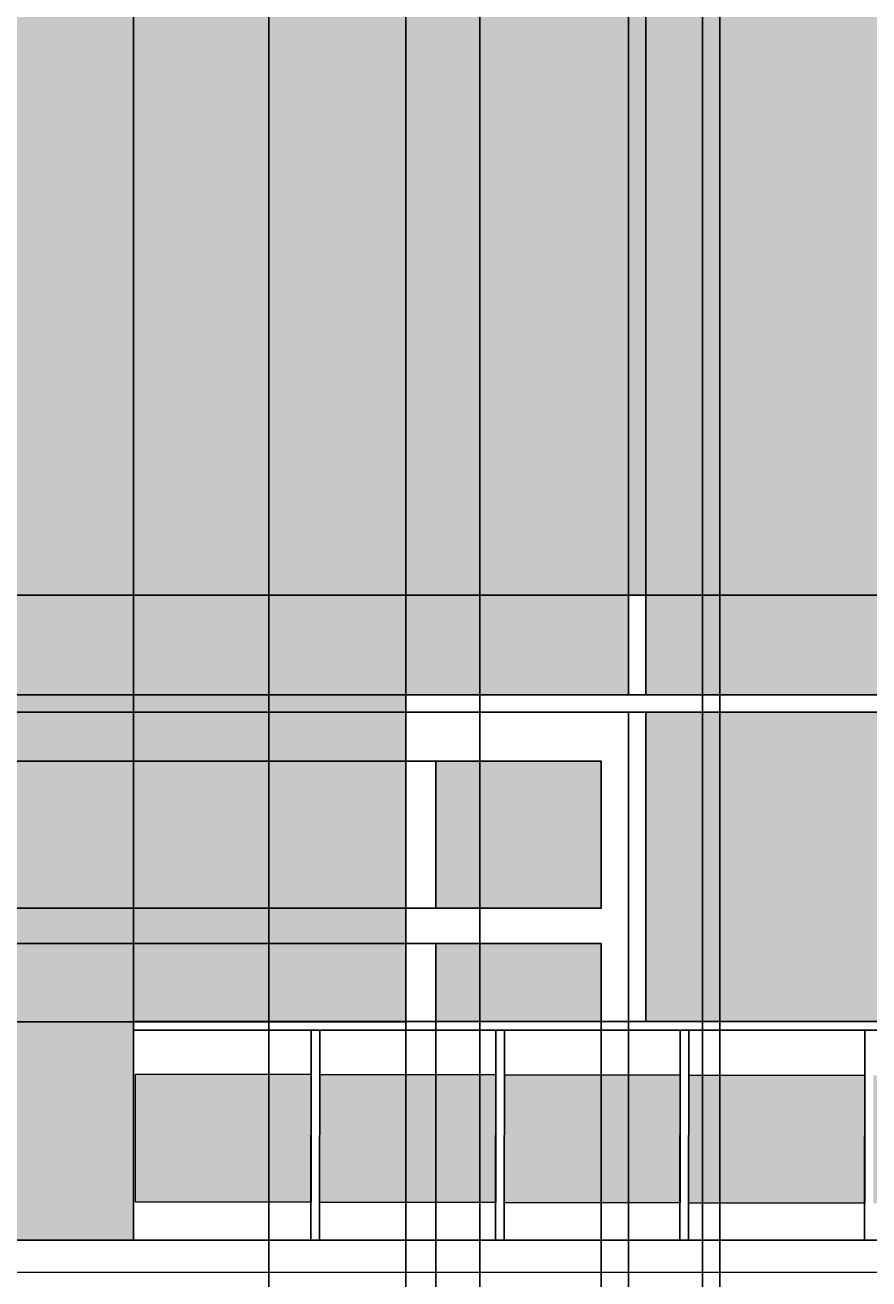
# Model space of a CAD drawing. Units: inches. Extents: x 36 to 594, y 79 to 831.
# Tile 18 of 30: x 189 to 286, y 446 to 590. Entities that reach past the tile are written whole.
import ezdxf

# ---------------------------------------------------------------- set-up
doc = ezdxf.new("R2010")
doc.units = ezdxf.units.IN
doc.header["$MEASUREMENT"] = 0
for name, color, linetype, lineweight in [('A-ANNO-DIMS', 2, 'Continuous', 18), ('A-ELEV', 7, 'Continuous', 25), ('A-ELEV-PATT', 8, 'Continuous', 13), ('A-GLAZ', 4, 'Continuous', 18)]:
    doc.layers.add(name, color=color, linetype=linetype, lineweight=lineweight)
doc.styles.get("Standard").update_dxf_attribs({"font": 'arial.ttf'})
doc.dimstyles.get("Standard").update_dxf_attribs({"dimtxt": 0.8125, "dimasz": 0.18, "dimexe": 0.18, "dimexo": 0.0625, "dimgap": 0.09, "dimtad": 0, "dimtih": 1, "dimtoh": 1, "dimdec": 4, "dimzin": 0, "dimdsep": 46, "dimlunit": 4, "dimtxsty": 'Standard', "dimcen": 0.09, "dimadec": 0, "dimazin": 0, "dimtfac": 1, "dimtdec": 4, "dimtofl": 0, "dimtmove": 0, "dimatfit": 3, "dimfxl": 1, "dimtolj": 1, "dimtzin": 0, "dimarcsym": 0})

# ---------------------------------------------------------------- blocks, each defined once
blk = doc.blocks.new('GLAZ-PANEL')
blk.add_lwpolyline([(0, 14.77), (20.28, 14.77), (20.28, 0), (0, 0)], close=True)
blk = doc.blocks.new('*D28')
at = {"layer": 'A-ANNO-DIMS', "color": 0, "lineweight": -2, "transparency": 16777216}
for p, q in [((269.3, 796.05), (37.49, 796.05)), ((37.67, 795.87), (37.67, 455.63)), ((37.67, 114.39), (37.67, 454.62)), ((94.8, 114.21), (37.49, 114.21))]:
    blk.add_line(p, q, dxfattribs=at)
at = {"layer": 'A-ANNO-DIMS', "color": 0, "transparency": 16777216}
for points in [[(37.64, 795.87), (37.7, 795.87), (37.67, 796.05)], [(37.64, 114.39), (37.7, 114.39), (37.67, 114.21)]]:
    blk.add_solid(points, dxfattribs=at)
at = {"layer": 'Defpoints', "color": 0, "transparency": 16777216}
for p in [(37.67, 796.05), (269.36, 796.05), (94.87, 114.21)]:
    blk.add_point(p, dxfattribs=at)
at = {"layer": 'A-ANNO-DIMS', "color": 0, "transparency": 16777216, "insert": (37.67, 455.13), "char_height": 0.812, "attachment_point": 5}
blk.add_mtext('\\A1;681.8', dxfattribs=at)
blk = doc.blocks.new('*D61')
at = {"layer": 'A-ANNO-DIMS', "color": 0, "lineweight": -2, "transparency": 16777216}
for p, q in [((156.41, 264.68), (156.41, 830.73)), ((156.59, 830.55), (185.26, 830.55)), ((216.85, 830.55), (188.18, 830.55)), ((217.03, 286.24), (217.03, 830.73))]:
    blk.add_line(p, q, dxfattribs=at)
at = {"layer": 'A-ANNO-DIMS', "color": 0, "transparency": 16777216}
for points in [[(156.59, 830.58), (156.59, 830.52), (156.41, 830.55)], [(216.85, 830.58), (216.85, 830.52), (217.03, 830.55)]]:
    blk.add_solid(points, dxfattribs=at)
at = {"layer": 'Defpoints', "color": 0, "transparency": 16777216}
for p in [(217.03, 830.55), (217.03, 286.18), (156.41, 264.62)]:
    blk.add_point(p, dxfattribs=at)
at = {"layer": 'A-ANNO-DIMS', "color": 0, "transparency": 16777216, "insert": (186.72, 830.55), "char_height": 0.812, "attachment_point": 5}
blk.add_mtext('\\A1;60.62', dxfattribs=at)
blk = doc.blocks.new('*D92')
at = {"layer": 'A-ANNO-DIMS', "color": 0, "lineweight": -2, "transparency": 16777216}
for p, q in [((201.42, 475.48), (201.42, 830.73)), ((201.6, 830.55), (215.98, 830.55)), ((232.64, 830.55), (218.26, 830.55)), ((232.82, 524.67), (232.82, 830.73))]:
    blk.add_line(p, q, dxfattribs=at)
at = {"layer": 'A-ANNO-DIMS', "color": 0, "transparency": 16777216}
for points in [[(201.6, 830.58), (201.6, 830.52), (201.42, 830.55)], [(232.64, 830.58), (232.64, 830.52), (232.82, 830.55)]]:
    blk.add_solid(points, dxfattribs=at)
at = {"layer": 'Defpoints', "color": 0, "transparency": 16777216}
for p in [(232.82, 830.55), (232.82, 524.6), (201.42, 475.41)]:
    blk.add_point(p, dxfattribs=at)
at = {"layer": 'A-ANNO-DIMS', "color": 0, "transparency": 16777216, "insert": (217.12, 830.55), "char_height": 0.812, "attachment_point": 5}
blk.add_mtext('\\A1;31.4', dxfattribs=at)
blk = doc.blocks.new('*D93')
at = {"layer": 'A-ANNO-DIMS', "color": 0, "lineweight": -2, "transparency": 16777216}
for p, q in [((232.82, 524.67), (232.82, 830.73)), ((233, 830.55), (243.88, 830.55)), ((258.33, 830.55), (247.45, 830.55)), ((258.51, 524.67), (258.51, 830.73))]:
    blk.add_line(p, q, dxfattribs=at)
at = {"layer": 'A-ANNO-DIMS', "color": 0, "transparency": 16777216}
for points in [[(233, 830.58), (233, 830.52), (232.82, 830.55)], [(258.33, 830.58), (258.33, 830.52), (258.51, 830.55)]]:
    blk.add_solid(points, dxfattribs=at)
at = {"layer": 'Defpoints', "color": 0, "transparency": 16777216}
for p in [(258.51, 830.55), (232.82, 524.6), (258.51, 524.6)]:
    blk.add_point(p, dxfattribs=at)
at = {"layer": 'A-ANNO-DIMS', "color": 0, "transparency": 16777216, "insert": (245.66, 830.55), "char_height": 0.812, "attachment_point": 5}
blk.add_mtext('\\A1;25.684', dxfattribs=at)
blk = doc.blocks.new('*D94')
at = {"layer": 'A-ANNO-DIMS', "color": 0, "lineweight": -2, "transparency": 16777216}
for p, q in [((258.51, 524.67), (258.51, 830.73)), ((258.69, 830.55), (259.15, 830.55)), ((260.33, 830.55), (259.86, 830.55)), ((260.51, 524.67), (260.51, 830.73))]:
    blk.add_line(p, q, dxfattribs=at)
at = {"layer": 'A-ANNO-DIMS', "color": 0, "transparency": 16777216}
for points in [[(258.69, 830.58), (258.69, 830.52), (258.51, 830.55)], [(260.33, 830.58), (260.33, 830.52), (260.51, 830.55)]]:
    blk.add_solid(points, dxfattribs=at)
at = {"layer": 'Defpoints', "color": 0, "transparency": 16777216}
for p in [(260.51, 830.55), (258.51, 524.6), (260.51, 524.6)]:
    blk.add_point(p, dxfattribs=at)
at = {"layer": 'A-ANNO-DIMS', "color": 0, "transparency": 16777216, "insert": (259.51, 830.55), "char_height": 0.812, "attachment_point": 5}
blk.add_mtext('\\A1;2', dxfattribs=at)
blk = doc.blocks.new('*D95')
at = {"layer": 'A-ANNO-DIMS', "color": 0, "lineweight": -2, "transparency": 16777216}
for p, q in [((260.51, 524.67), (260.51, 830.73)), ((260.69, 830.55), (299.71, 830.55)), ((341.66, 830.55), (302.63, 830.55)), ((341.84, 524.67), (341.84, 830.73))]:
    blk.add_line(p, q, dxfattribs=at)
at = {"layer": 'A-ANNO-DIMS', "color": 0, "transparency": 16777216}
for points in [[(260.69, 830.58), (260.69, 830.52), (260.51, 830.55)], [(341.66, 830.58), (341.66, 830.52), (341.84, 830.55)]]:
    blk.add_solid(points, dxfattribs=at)
at = {"layer": 'Defpoints', "color": 0, "transparency": 16777216}
for p in [(341.84, 830.55), (260.51, 524.6), (341.84, 524.6)]:
    blk.add_point(p, dxfattribs=at)
at = {"layer": 'A-ANNO-DIMS', "color": 0, "transparency": 16777216, "insert": (301.17, 830.55), "char_height": 0.812, "attachment_point": 5}
blk.add_mtext('\\A1;81.33', dxfattribs=at)
blk = doc.blocks.new('*D96')
at = {"layer": 'A-ANNO-DIMS', "color": 0, "lineweight": -2, "transparency": 16777216}
for p, q in [((236.29, 484.36), (236.29, 79.53)), ((232.82, 475.35), (232.82, 79.53)), ((233, 79.71), (233.41, 79.71)), ((236.11, 79.71), (235.7, 79.71))]:
    blk.add_line(p, q, dxfattribs=at)
at = {"layer": 'A-ANNO-DIMS', "color": 0, "transparency": 16777216}
for points in [[(233, 79.74), (233, 79.68), (232.82, 79.71)], [(236.11, 79.74), (236.11, 79.68), (236.29, 79.71)]]:
    blk.add_solid(points, dxfattribs=at)
at = {"layer": 'Defpoints', "color": 0, "transparency": 16777216}
for p in [(236.29, 484.42), (232.82, 475.41), (236.29, 79.71)]:
    blk.add_point(p, dxfattribs=at)
at = {"layer": 'A-ANNO-DIMS', "color": 0, "transparency": 16777216, "insert": (234.56, 79.71), "char_height": 0.812, "attachment_point": 5}
blk.add_mtext('\\A1;3.47', dxfattribs=at)
blk = doc.blocks.new('*D97')
at = {"layer": 'A-ANNO-DIMS', "color": 0, "lineweight": -2, "transparency": 16777216}
for p, q in [((236.29, 484.36), (236.29, 79.53)), ((255.36, 484.36), (255.36, 79.53)), ((236.47, 79.71), (244.09, 79.71)), ((255.18, 79.71), (247.56, 79.71))]:
    blk.add_line(p, q, dxfattribs=at)
at = {"layer": 'A-ANNO-DIMS', "color": 0, "transparency": 16777216}
for points in [[(236.47, 79.74), (236.47, 79.68), (236.29, 79.71)], [(255.18, 79.74), (255.18, 79.68), (255.36, 79.71)]]:
    blk.add_solid(points, dxfattribs=at)
at = {"layer": 'Defpoints', "color": 0, "transparency": 16777216}
for p in [(236.29, 484.42), (255.36, 484.42), (255.36, 79.71)]:
    blk.add_point(p, dxfattribs=at)
at = {"layer": 'A-ANNO-DIMS', "color": 0, "transparency": 16777216, "insert": (245.82, 79.71), "char_height": 0.812, "attachment_point": 5}
blk.add_mtext('\\A1;19.064', dxfattribs=at)
blk = doc.blocks.new('*D98')
at = {"layer": 'A-ANNO-DIMS', "color": 0, "lineweight": -2, "transparency": 16777216}
for p, q in [((255.36, 484.36), (255.36, 79.53)), ((258.51, 475.35), (258.51, 79.53)), ((255.54, 79.71), (255.78, 79.71)), ((258.33, 79.71), (258.08, 79.71))]:
    blk.add_line(p, q, dxfattribs=at)
at = {"layer": 'A-ANNO-DIMS', "color": 0, "transparency": 16777216}
for points in [[(255.54, 79.74), (255.54, 79.68), (255.36, 79.71)], [(258.33, 79.74), (258.33, 79.68), (258.51, 79.71)]]:
    blk.add_solid(points, dxfattribs=at)
at = {"layer": 'Defpoints', "color": 0, "transparency": 16777216}
for p in [(255.36, 484.42), (258.51, 475.41), (258.51, 79.71)]:
    blk.add_point(p, dxfattribs=at)
at = {"layer": 'A-ANNO-DIMS', "color": 0, "transparency": 16777216, "insert": (256.93, 79.71), "char_height": 0.812, "attachment_point": 5}
blk.add_mtext('\\A1;3.15', dxfattribs=at)
blk = doc.blocks.new('*D99')
at = {"layer": 'A-ANNO-DIMS', "color": 0, "lineweight": -2, "transparency": 16777216}
for p, q in [((236.23, 484.42), (37.49, 484.42)), ((37.67, 484.24), (37.67, 480.42)), ((37.67, 475.59), (37.67, 479.41)), ((232.76, 475.41), (37.49, 475.41))]:
    blk.add_line(p, q, dxfattribs=at)
at = {"layer": 'A-ANNO-DIMS', "color": 0, "transparency": 16777216}
for points in [[(37.64, 484.24), (37.7, 484.24), (37.67, 484.42)], [(37.64, 475.59), (37.7, 475.59), (37.67, 475.41)]]:
    blk.add_solid(points, dxfattribs=at)
at = {"layer": 'Defpoints', "color": 0, "transparency": 16777216}
for p in [(37.67, 484.42), (236.29, 484.42), (232.82, 475.41)]:
    blk.add_point(p, dxfattribs=at)
at = {"layer": 'A-ANNO-DIMS', "color": 0, "transparency": 16777216, "insert": (37.67, 479.92), "char_height": 0.812, "attachment_point": 5}
blk.add_mtext('\\A1;9.005', dxfattribs=at)
blk = doc.blocks.new('*D100')
at = {"layer": 'A-ANNO-DIMS', "color": 0, "lineweight": -2, "transparency": 16777216}
for p, q in [((236.23, 488.49), (37.49, 488.49)), ((37.67, 488.31), (37.67, 486.96)), ((37.67, 484.6), (37.67, 485.95)), ((236.23, 484.42), (37.49, 484.42))]:
    blk.add_line(p, q, dxfattribs=at)
at = {"layer": 'A-ANNO-DIMS', "color": 0, "transparency": 16777216}
for points in [[(37.64, 488.31), (37.7, 488.31), (37.67, 488.49)], [(37.64, 484.6), (37.7, 484.6), (37.67, 484.42)]]:
    blk.add_solid(points, dxfattribs=at)
at = {"layer": 'Defpoints', "color": 0, "transparency": 16777216}
for p in [(37.67, 488.49), (236.29, 488.49), (236.29, 484.42)]:
    blk.add_point(p, dxfattribs=at)
at = {"layer": 'A-ANNO-DIMS', "color": 0, "transparency": 16777216, "insert": (37.67, 486.46), "char_height": 0.812, "attachment_point": 5}
blk.add_mtext('\\A1;4.074', dxfattribs=at)
blk = doc.blocks.new('*D101')
at = {"layer": 'A-ANNO-DIMS', "color": 0, "lineweight": -2, "transparency": 16777216}
for p, q in [((236.23, 505.45), (37.49, 505.45)), ((37.67, 505.27), (37.67, 497.48)), ((37.67, 488.67), (37.67, 496.47)), ((236.23, 488.49), (37.49, 488.49))]:
    blk.add_line(p, q, dxfattribs=at)
at = {"layer": 'A-ANNO-DIMS', "color": 0, "transparency": 16777216}
for points in [[(37.64, 505.27), (37.7, 505.27), (37.67, 505.45)], [(37.64, 488.67), (37.7, 488.67), (37.67, 488.49)]]:
    blk.add_solid(points, dxfattribs=at)
at = {"layer": 'Defpoints', "color": 0, "transparency": 16777216}
for p in [(37.67, 505.45), (236.29, 505.45), (236.29, 488.49)]:
    blk.add_point(p, dxfattribs=at)
at = {"layer": 'A-ANNO-DIMS', "color": 0, "transparency": 16777216, "insert": (37.67, 496.97), "char_height": 0.812, "attachment_point": 5}
blk.add_mtext('\\A1;16.957', dxfattribs=at)
blk = doc.blocks.new('*D102')
at = {"layer": 'A-ANNO-DIMS', "color": 0, "lineweight": -2, "transparency": 16777216}
for p, q in [((232.76, 511.12), (37.49, 511.12)), ((37.67, 510.94), (37.67, 508.79)), ((37.67, 505.63), (37.67, 507.78)), ((236.23, 505.45), (37.49, 505.45))]:
    blk.add_line(p, q, dxfattribs=at)
at = {"layer": 'A-ANNO-DIMS', "color": 0, "transparency": 16777216}
for points in [[(37.64, 510.94), (37.7, 510.94), (37.67, 511.12)], [(37.64, 505.63), (37.7, 505.63), (37.67, 505.45)]]:
    blk.add_solid(points, dxfattribs=at)
at = {"layer": 'Defpoints', "color": 0, "transparency": 16777216}
for p in [(37.67, 511.12), (232.82, 511.12), (236.29, 505.45)]:
    blk.add_point(p, dxfattribs=at)
at = {"layer": 'A-ANNO-DIMS', "color": 0, "transparency": 16777216, "insert": (37.67, 508.29), "char_height": 0.812, "attachment_point": 5}
blk.add_mtext('\\A1;5.672', dxfattribs=at)
blk = doc.blocks.new('*D103')
at = {"layer": 'A-ANNO-DIMS', "color": 0, "lineweight": -2, "transparency": 16777216}
for p, q in [((232.76, 513.12), (37.49, 513.12)), ((37.67, 512.94), (37.67, 512.62)), ((232.76, 511.12), (37.49, 511.12)), ((37.67, 511.3), (37.67, 511.62))]:
    blk.add_line(p, q, dxfattribs=at)
at = {"layer": 'A-ANNO-DIMS', "color": 0, "transparency": 16777216}
for points in [[(37.64, 512.94), (37.7, 512.94), (37.67, 513.12)], [(37.64, 511.3), (37.7, 511.3), (37.67, 511.12)]]:
    blk.add_solid(points, dxfattribs=at)
at = {"layer": 'Defpoints', "color": 0, "transparency": 16777216}
for p in [(37.67, 513.12), (232.82, 513.12), (232.82, 511.12)]:
    blk.add_point(p, dxfattribs=at)
at = {"layer": 'A-ANNO-DIMS', "color": 0, "transparency": 16777216, "insert": (37.67, 512.12), "char_height": 0.812, "attachment_point": 5}
blk.add_mtext('\\A1;2', dxfattribs=at)
blk = doc.blocks.new('*D104')
at = {"layer": 'A-ANNO-DIMS', "color": 0, "lineweight": -2, "transparency": 16777216}
for p, q in [((232.76, 524.6), (37.49, 524.6)), ((37.67, 524.42), (37.67, 519.37)), ((37.67, 513.3), (37.67, 518.36)), ((232.76, 513.12), (37.49, 513.12))]:
    blk.add_line(p, q, dxfattribs=at)
at = {"layer": 'A-ANNO-DIMS', "color": 0, "transparency": 16777216}
for points in [[(37.64, 524.42), (37.7, 524.42), (37.67, 524.6)], [(37.64, 513.3), (37.7, 513.3), (37.67, 513.12)]]:
    blk.add_solid(points, dxfattribs=at)
at = {"layer": 'Defpoints', "color": 0, "transparency": 16777216}
for p in [(37.67, 524.6), (232.82, 524.6), (232.82, 513.12)]:
    blk.add_point(p, dxfattribs=at)
at = {"layer": 'A-ANNO-DIMS', "color": 0, "transparency": 16777216, "insert": (37.67, 518.86), "char_height": 0.812, "attachment_point": 5}
blk.add_mtext('\\A1;11.481', dxfattribs=at)
blk = doc.blocks.new('*D105')
at = {"layer": 'A-ANNO-DIMS', "color": 0, "lineweight": -2, "transparency": 16777216}
for p, q in [((241.36, 404.34), (241.36, 830.73)), ((241.54, 830.55), (252.42, 830.55)), ((266.86, 830.55), (255.98, 830.55)), ((267.04, 404.34), (267.04, 830.73))]:
    blk.add_line(p, q, dxfattribs=at)
at = {"layer": 'A-ANNO-DIMS', "color": 0, "transparency": 16777216}
for points in [[(241.54, 830.58), (241.54, 830.52), (241.36, 830.55)], [(266.86, 830.58), (266.86, 830.52), (267.04, 830.55)]]:
    blk.add_solid(points, dxfattribs=at)
at = {"layer": 'Defpoints', "color": 0, "transparency": 16777216}
for p in [(267.04, 830.55), (241.36, 404.27), (267.04, 404.27)]:
    blk.add_point(p, dxfattribs=at)
at = {"layer": 'A-ANNO-DIMS', "color": 0, "transparency": 16777216, "insert": (254.2, 830.55), "char_height": 0.812, "attachment_point": 5}
blk.add_mtext('\\A1;25.684', dxfattribs=at)
blk = doc.blocks.new('*D106')
at = {"layer": 'A-ANNO-DIMS', "color": 0, "lineweight": -2, "transparency": 16777216}
for p, q in [((267.04, 404.34), (267.04, 830.73)), ((267.22, 830.55), (267.68, 830.55)), ((268.86, 830.55), (268.4, 830.55)), ((269.04, 404.34), (269.04, 830.73))]:
    blk.add_line(p, q, dxfattribs=at)
at = {"layer": 'A-ANNO-DIMS', "color": 0, "transparency": 16777216}
for points in [[(267.22, 830.58), (267.22, 830.52), (267.04, 830.55)], [(268.86, 830.58), (268.86, 830.52), (269.04, 830.55)]]:
    blk.add_solid(points, dxfattribs=at)
at = {"layer": 'Defpoints', "color": 0, "transparency": 16777216}
for p in [(269.04, 830.55), (267.04, 404.27), (269.04, 404.27)]:
    blk.add_point(p, dxfattribs=at)
at = {"layer": 'A-ANNO-DIMS', "color": 0, "transparency": 16777216, "insert": (268.04, 830.55), "char_height": 0.812, "attachment_point": 5}
blk.add_mtext('\\A1;2', dxfattribs=at)
blk = doc.blocks.new('*D107')
at = {"layer": 'A-ANNO-DIMS', "color": 0, "lineweight": -2, "transparency": 16777216}
for p, q in [((269.04, 404.34), (269.04, 830.73)), ((269.22, 830.55), (310.99, 830.55)), ((355.68, 830.55), (313.91, 830.55)), ((355.86, 404.34), (355.86, 830.73))]:
    blk.add_line(p, q, dxfattribs=at)
at = {"layer": 'A-ANNO-DIMS', "color": 0, "transparency": 16777216}
for points in [[(269.22, 830.58), (269.22, 830.52), (269.04, 830.55)], [(355.68, 830.58), (355.68, 830.52), (355.86, 830.55)]]:
    blk.add_solid(points, dxfattribs=at)
at = {"layer": 'Defpoints', "color": 0, "transparency": 16777216}
for p in [(355.86, 830.55), (269.04, 404.27), (355.86, 404.27)]:
    blk.add_point(p, dxfattribs=at)
at = {"layer": 'A-ANNO-DIMS', "color": 0, "transparency": 16777216, "insert": (312.45, 830.55), "char_height": 0.812, "attachment_point": 5}
blk.add_mtext('\\A1;86.82', dxfattribs=at)

msp = doc.modelspace()

# ---------------------------------------------------------------- hatches: boundary and pattern name
at = {"layer": 'A-ELEV-PATT'}
h = msp.add_hatch(color=256, dxfattribs=at)
h.dxf.hatch_style = 1
h.paths.add_polyline_path([(398.0873, 796.0465), (269.3592, 796.0465), (269.3592, 770.1455), (397.8159, 770.1455)])
h.paths.add_polyline_path([(397.7518, 764.0341), (269.3592, 764.0341), (269.3592, 630.0394), (341.8367, 630.0394), (341.8367, 720.595), (335.0881, 728.3699), (329.982, 735.3373), (345.3661, 727.7743), (397.1052, 702.3389)])
h.paths.add_polyline_path([(341.8367, 594.2124), (201.4189, 594.2124), (201.4189, 475.4136), (232.8216, 475.4136), (232.8216, 524.6037), (341.8367, 524.6037)])
h.paths.add_polyline_path([(177.525, 594.2124), (118.7598, 594.2124), (118.7598, 450.2124), (177.525, 450.2124)])
h.paths.add_polyline_path([(424.4958, 594.2124), (365.7306, 594.2124), (365.7306, 450.2124), (424.4958, 450.2124)])
h.paths.add_polyline_path([(241.3553, 404.2737), (355.8569, 404.2737), (355.8569, 355.0836), (424.5492, 355.0836), (424.5492, 425.7333), (118.7598, 426.2844), (118.7598, 355.0836), (241.3553, 355.0836)])
h.paths.add_polyline_path([(448.3898, 306.2124), (217.0273, 306.2124), (217.0273, 142.2124), (254.0293, 142.2124), (254.0293, 150.9347), (254.0293, 286.1802), (401.5491, 286.1802), (401.5491, 150.9347), (401.5491, 142.2124), (448.3898, 142.2124)])
h.paths.add_polyline_path([(448.3898, 142.2124), (401.5491, 142.2124), (217.0273, 142.2124), (217.0273, 114.2124), (448.3898, 114.2124)])
h.paths.add_polyline_path([(217.0273, 306.2124), (174.7353, 306.2124), (94.8658, 306.2124), (94.8658, 162.2124), (103.3368, 162.2124), (103.3368, 264.6224), (103.3368, 286.1802), (217.0273, 286.1802)])
h = msp.add_hatch(color=256, dxfattribs=at)
h.dxf.hatch_style = 1
h.paths.add_polyline_path([(448.3898, 668.2124), (341.8367, 720.595), (341.8367, 594.2124), (341.8367, 450.2124), (365.7306, 450.2124), (365.7306, 594.2124), (424.4958, 594.2124), (424.4958, 450.2124), (448.3898, 450.2124), (448.3898, 594.2124)])
h.paths.add_polyline_path([(378.5958, 653.8563, -1), (413.2033, 653.8563, -1)], flags=16)
h.paths.add_polyline_path([(394.8995, 653.8563), (394.8995, 654.8563), (395.8995, 654.8563), (396.8995, 654.8563), (396.8995, 653.8563), (396.8995, 652.8563), (395.8995, 652.8563), (394.8995, 652.8563)], flags=0)
h.paths.add_polyline_path([(201.4189, 708.8485), (201.4189, 720.595), (94.8658, 668.2124), (94.8658, 644.2124), (94.8658, 596.2124), (94.8658, 594.2124), (94.8658, 450.2124), (118.7598, 450.2124), (118.7598, 594.2124), (177.525, 594.2124), (177.525, 450.2124), (201.4189, 450.2124), (201.4189, 594.2124)])
h.paths.add_polyline_path([(130.1589, 653.7648, -1), (164.7665, 653.7648, -1)], flags=16)
h.paths.add_polyline_path([(148.4627, 652.7648), (147.4627, 652.7648), (146.4627, 652.7648), (146.4627, 653.7648), (146.4627, 654.7648), (147.4627, 654.7648), (148.4627, 654.7648), (148.4627, 653.7648)], flags=0)
h = msp.add_hatch(color=256, dxfattribs=at)
h.dxf.hatch_style = 1
h.set_gradient(color1=(0, 255, 255), color2=(16, 86, 137))
h.paths.add_polyline_path([(341.8367, 524.6037), (260.5056, 524.6037), (260.5056, 513.1224), (341.8367, 513.1224)])
h.paths.add_polyline_path([(341.8367, 511.1224), (260.5056, 511.1224), (260.5056, 475.4136), (341.8367, 475.4136)])
h.paths.add_polyline_path([(258.5056, 524.6037), (232.8216, 524.6037), (232.8216, 513.1224), (258.5056, 513.1224)])
h.paths.add_polyline_path([(355.8569, 404.2737), (269.0393, 404.2737), (269.0393, 392.7924), (355.8569, 392.7924)])
h.paths.add_polyline_path([(267.0393, 404.2737), (241.3553, 404.2737), (241.3553, 392.7924), (267.0393, 392.7924)])
h.paths.add_polyline_path([(355.8569, 390.7924), (269.0393, 390.7924), (269.0393, 355.0836), (355.8569, 355.0836)])
h.paths.add_polyline_path([(399.5491, 284.1802), (256.0293, 284.1802), (256.0293, 271.378), (399.5491, 271.378)])
h.paths.add_polyline_path([(317.3533, 259.1243), (262.3169, 259.1243), (262.3169, 200.6645), (317.3533, 200.6645)])
h.paths.add_polyline_path([(390.386, 259.1243), (335.3496, 259.1243), (335.3496, 200.6645), (390.386, 200.6645)])
h.paths.add_polyline_path([(390.386, 190.7697), (335.3496, 190.7697), (335.3496, 162.9881), (390.386, 162.9881)])
h.paths.add_polyline_path([(317.3533, 190.7697), (262.3169, 190.7697), (262.3169, 162.9881), (317.3533, 162.9881)])
h.paths.add_polyline_path([(215.0273, 262.6224), (158.4069, 262.6224), (158.4069, 181.4195), (215.0273, 181.4195)])
h.paths.add_polyline_path([(215.0273, 284.1802), (105.3368, 284.1802), (105.3368, 266.6224), (215.0273, 266.6224)])
h = msp.add_hatch(dxfattribs=at)
h.set_pattern_fill('ANSI33', color=256, scale=6.3, angle=135)
h.paths.add_polyline_path([(255.3555, 505.4499), (236.2911, 505.4499), (236.2911, 488.4928), (255.3555, 488.4928)])
h.paths.add_polyline_path([(255.3555, 484.4187), (236.2911, 484.4187), (236.2911, 475.4136), (255.3555, 475.4136)])
h.paths.add_polyline_path([(263.8892, 385.1199), (244.8248, 385.1199), (244.8248, 368.1628), (263.8892, 368.1628)])
h.paths.add_polyline_path([(263.8892, 364.0887), (244.8248, 364.0887), (244.8248, 355.0836), (263.8892, 355.0836)])
h.paths.add_polyline_path([(148.0383, 248.8663), (113.6593, 248.8663), (113.6593, 214.2237), (148.0383, 214.2237)])
h.paths.add_polyline_path([(148.0383, 203.057), (113.6593, 203.057), (113.6593, 170.5978), (148.0383, 170.5978)])
h = msp.add_hatch(color=256, dxfattribs=at)
h.dxf.hatch_style = 1
h.set_gradient(color1=(192, 192, 192), color2=(0, 0, 0))
h.paths.add_polyline_path([(243.19, 469.3251), (222.9132, 469.3251), (222.9132, 454.5571), (243.1634, 454.5571)])
h.paths.add_polyline_path([(264.4667, 469.2868), (244.1899, 469.2868), (244.1899, 454.5188), (264.4401, 454.5188)])
h.paths.add_polyline_path([(285.7435, 469.2484), (265.4667, 469.2484), (265.4667, 454.4804), (285.7168, 454.4804)])
h.paths.add_polyline_path([(307.0202, 469.2101), (286.7434, 469.2101), (286.7434, 454.4421), (306.9936, 454.4421)])
h.paths.add_polyline_path([(328.2969, 469.1717), (308.0201, 469.1717), (308.0201, 454.4037), (328.2703, 454.4037)])
h.paths.add_polyline_path([(341.8367, 469.1334), (329.2969, 469.1334), (329.2969, 454.3654), (341.8367, 454.3654)])
h.paths.add_polyline_path([(221.9133, 469.3635), (201.6365, 469.3635), (201.6365, 454.5955), (221.8866, 454.5955)])
h.paths.add_polyline_path([(145.3401, 349.1868), (125.0633, 349.1868), (125.0633, 334.4189), (145.3134, 334.4189)])
h.paths.add_polyline_path([(166.6168, 349.1485), (146.34, 349.1485), (146.34, 334.3805), (166.5902, 334.3805)])
h.paths.add_polyline_path([(187.8935, 349.1101), (167.6167, 349.1101), (167.6167, 334.3422), (187.8669, 334.3422)])
h.paths.add_polyline_path([(209.1703, 349.0718), (188.8935, 349.0718), (188.8935, 334.3038), (209.1436, 334.3038)])
h.paths.add_polyline_path([(230.447, 349.0335), (210.1702, 349.0335), (210.1702, 334.2655), (230.4204, 334.2655)])
h.paths.add_polyline_path([(251.7237, 348.9951), (231.4469, 348.9951), (231.4469, 334.2271), (251.6971, 334.2271)])
h.paths.add_polyline_path([(273.0005, 348.9568), (252.7236, 348.9568), (252.7236, 334.1888), (272.9738, 334.1888)])
h.paths.add_polyline_path([(294.2772, 348.9184), (274.0004, 348.9184), (274.0004, 334.1504), (294.2506, 334.1504)])
h.paths.add_polyline_path([(315.5539, 348.8801), (295.2771, 348.8801), (295.2771, 334.1121), (315.5273, 334.1121)])
h.paths.add_polyline_path([(336.8306, 348.8417), (316.5538, 348.8417), (316.5538, 334.0737), (336.804, 334.0737)])
h.paths.add_polyline_path([(358.1074, 348.8034), (337.8306, 348.8034), (337.8306, 334.0354), (358.0808, 334.0354)])
h.paths.add_polyline_path([(379.3841, 348.765), (359.1073, 348.765), (359.1073, 333.997), (379.3575, 333.997)])
h.paths.add_polyline_path([(400.6608, 348.7267), (380.384, 348.7267), (380.384, 333.9587), (400.6342, 333.9587)])
h.paths.add_polyline_path([(421.9376, 348.6883), (401.6608, 348.6883), (401.6608, 333.9204), (421.911, 333.9204)])
h.paths.add_polyline_path([(103.3368, 162.2124), (94.8658, 162.2124), (94.8658, 150.2124), (94.8658, 114.2124), (103.3368, 114.2124)])
h.paths.add_polyline_path([(217.0273, 132.2124), (103.3368, 132.2124), (103.3368, 122.2124), (217.0273, 122.2124)])
h.paths.add_polyline_path([(217.0273, 122.2124), (103.3368, 122.2124), (103.3368, 114.2124), (217.0273, 114.2124)])
h.paths.add_polyline_path([(217.0273, 142.2124), (174.7353, 142.2124), (103.3368, 142.2124), (103.3368, 132.2124), (217.0273, 132.2124)])
h.paths.add_polyline_path([(217.0273, 152.2124), (103.3368, 152.2124), (103.3368, 142.2124), (174.7353, 142.2124), (217.0273, 142.2124)])
h.paths.add_polyline_path([(217.0273, 162.2124), (103.3368, 162.2124), (103.3368, 152.2124), (217.0273, 152.2124)])
h = msp.add_hatch(dxfattribs=at)
h.set_pattern_fill('ANSI31', color=256, scale=38, angle=135)
h.paths.add_polyline_path([(448.3898, 450.2124), (94.8658, 450.2124), (94.8658, 306.2124), (174.7353, 306.2124), (448.3898, 306.2124), (448.3898, 367.5118)])
h.paths.add_polyline_path([(424.5492, 425.7333), (424.5492, 329.5325), (118.7598, 330.0836), (118.7598, 354.0836), (118.7598, 426.2844)], flags=16)
h.paths.add_polyline_path([(355.8569, 404.2737), (355.8569, 355.0836), (241.3553, 355.0836), (241.3553, 404.2737)], flags=0)
h.paths.add_polyline_path([(269.0393, 390.7924), (269.0393, 355.0836), (244.8248, 355.0836), (244.8248, 364.0887), (263.8892, 364.0887), (263.8892, 355.0836), (267.0393, 355.0836), (267.0393, 390.7924)], flags=0)
h.paths.add_polyline_path([(303.9765, 436.9126, -1), (313.1496, 436.9126, -1)], flags=16)
h.paths.add_polyline_path([(421.9473, 354.0836), (421.9376, 348.6883), (421.9376, 333.9204), (401.6342, 333.9204), (401.6705, 354.0836), (400.6705, 354.0836), (400.6608, 348.7267), (400.6608, 333.9587), (380.3574, 333.9587), (380.3937, 354.0836), (379.3937, 354.0836), (379.3841, 348.765), (379.3841, 333.997), (359.0807, 333.997), (359.1169, 354.0836), (358.1169, 354.0836), (358.1074, 348.8034), (358.1074, 334.0354), (337.804, 334.0354), (337.8401, 354.0836), (336.8401, 354.0836), (336.8306, 348.8417), (336.8306, 334.0737), (316.5272, 334.0737), (316.5633, 354.0836), (315.5633, 354.0836), (315.5539, 348.8801), (315.5539, 334.1121), (295.2505, 334.1121), (295.2865, 354.0836), (294.2865, 354.0836), (294.2772, 348.9184), (294.2772, 334.1504), (273.9738, 334.1504), (274.0097, 354.0836), (273.0097, 354.0836), (273.0005, 348.9568), (273.0005, 334.1888), (252.697, 334.1888), (252.7329, 354.0836), (251.7329, 354.0836), (251.7237, 348.9951), (251.7237, 334.2271), (231.4203, 334.2271), (231.4561, 354.0836), (230.4561, 354.0836), (230.447, 349.0335), (230.447, 334.2655), (210.1436, 334.2655), (210.1793, 354.0836), (209.1793, 354.0836), (209.1703, 349.0718), (209.1703, 334.3038), (188.8668, 334.3038), (188.9025, 354.0836), (187.9025, 354.0836), (187.8935, 349.1101), (187.8935, 334.3422), (167.5901, 334.3422), (167.6257, 354.0836), (166.6257, 354.0836), (166.6168, 349.1485), (166.6168, 334.3805), (146.3134, 334.3805), (146.3489, 354.0836), (145.3489, 354.0836), (145.3401, 349.1868), (145.3401, 334.4189), (125.0366, 334.4189), (125.0721, 354.0836)], flags=0)
h.paths.add_polyline_path([(266.285, 436.9126, -1), (275.458, 436.9126, -1)], flags=16)
h.paths.add_polyline_path([(367.0204, 316.8739, -1), (357.8474, 316.8739, -1)], flags=16)
h.paths.add_polyline_path([(347.6933, 316.8739, -1), (338.5202, 316.8739, -1)], flags=16)
h.paths.add_polyline_path([(329.574, 316.8739, -1), (320.401, 316.8739, -1)], flags=16)
h.paths.add_polyline_path([(263.8892, 385.1199), (263.8892, 368.1628), (244.8248, 368.1628), (244.8248, 385.1199)], flags=0)
h.paths.add_polyline_path([(216.2543, 436.9126, -1), (225.4274, 436.9126, -1)], flags=16)
h.paths.add_polyline_path([(275.458, 316.8739, -1), (266.285, 316.8739, -1)], flags=16)
h.paths.add_polyline_path([(225.4274, 316.8739, -1), (216.2543, 316.8739, -1)], flags=16)

# ---------------------------------------------------------------- linework, layer by layer
at = {"layer": 'A-ELEV'}
for p, q in [((201.4189, 450.2124), (201.4189, 594.2124)), ((258.5056, 513.1224), (258.5056, 524.6037)), ((260.5056, 513.1224), (260.5056, 524.6037)), ((232.8216, 513.1224), (341.8367, 513.1224)), ((232.8216, 511.1224), (341.8367, 511.1224)), ((258.5056, 511.1224), (258.5056, 475.4136)), ((260.5056, 511.1224), (260.5056, 475.4136)), ((201.4189, 475.4136), (341.8367, 475.4136)), ((201.4189, 474.4136), (341.8367, 474.4136)), ((221.9224, 474.4136), (221.8788, 450.2507)), ((222.9224, 474.4136), (222.8788, 450.2489)), ((243.1992, 474.4136), (243.1555, 450.2124)), ((244.1992, 474.4136), (244.1555, 450.2106)), ((264.476, 474.4136), (264.4323, 450.174)), ((265.476, 474.4136), (265.4323, 450.1722)), ((285.7528, 474.4136), (285.709, 450.1357)), ((94.8658, 450.2124), (448.3898, 450.2124))]:
    msp.add_line(p, q, dxfattribs=at)
for points in [[(232.8216, 524.6037), (341.8367, 524.6037), (341.8367, 475.4136), (232.8216, 475.4136)], [(236.2911, 505.4499), (255.3555, 505.4499), (255.3555, 488.4928), (236.2911, 488.4928)], [(236.2911, 484.4187), (255.3555, 484.4187), (255.3555, 475.4136), (236.2911, 475.4136)]]:
    msp.add_lwpolyline(points, close=True, dxfattribs=at)

# ---------------------------------------------------------------- block references
at = {"layer": 'A-GLAZ'}
for p in [(201.6362, 454.5956), (222.9129, 454.5573), (244.1897, 454.5189), (265.4664, 454.4806)]:
    msp.add_blockref('GLAZ-PANEL', p, dxfattribs=at)

# ---------------------------------------------------------------- dimensions: what is measured, and where the dimension line sits
at = {"layer": 'A-ANNO-DIMS'}
for base, p1, p2, override, picture, middle in [((217.0273, 830.5465), (156.4069, 264.6224), (217.0273, 286.1802), {"dimdec": 2, "dimlfac": 1, "dimrnd": 0, "dimzin": 0, "dimdsep": 46, "dimlunit": 2}, '*D61', (186.7171, 830.5465)), ((232.8216, 830.5465), (201.4189, 475.4136), (232.8216, 524.6037), {"dimdec": 1, "dimlfac": 1, "dimrnd": 0, "dimzin": 0, "dimdsep": 46, "dimlunit": 2}, '*D92', (217.1202, 830.5465)), ((258.5056, 830.5465), (232.8216, 524.6037), (258.5056, 524.6037), {"dimdec": 3, "dimlfac": 1, "dimrnd": 0, "dimzin": 0, "dimdsep": 46, "dimlunit": 2}, '*D93', (245.6636, 830.5465)), ((267.0393, 830.5465), (241.3553, 404.2737), (267.0393, 404.2737), {"dimdec": 3, "dimlfac": 1, "dimrnd": 0, "dimzin": 0, "dimdsep": 46, "dimlunit": 2}, '*D105', (254.1973, 830.5465)), ((260.5056, 830.5465), (258.5056, 524.6037), (260.5056, 524.6037), {"dimdec": 0, "dimlfac": 1, "dimrnd": 0, "dimzin": 0, "dimdsep": 46, "dimlunit": 2}, '*D94', (259.5056, 830.5465)), ((341.8367, 830.5465), (260.5056, 524.6037), (341.8367, 524.6037), {"dimdec": 2, "dimlfac": 1, "dimrnd": 0, "dimzin": 0, "dimdsep": 46, "dimlunit": 2}, '*D95', (301.1711, 830.5465)), ((269.0393, 830.5465), (267.0393, 404.2737), (269.0393, 404.2737), {"dimdec": 0, "dimlfac": 1, "dimrnd": 0, "dimzin": 0, "dimdsep": 46, "dimlunit": 2}, '*D106', (268.0393, 830.5465)), ((355.8569, 830.5465), (269.0393, 404.2737), (355.8569, 404.2737), {"dimdec": 2, "dimlfac": 1, "dimrnd": 0, "dimzin": 0, "dimdsep": 46, "dimlunit": 2}, '*D107', (312.4481, 830.5465)), ((236.2911, 79.7124), (232.8216, 475.4136), (236.2911, 484.4187), {"dimdec": 2, "dimlfac": 1, "dimrnd": 0, "dimzin": 0, "dimdsep": 46, "dimlunit": 2}, '*D96', (234.5563, 79.7124)), ((255.3555, 79.7124), (236.2911, 484.4187), (255.3555, 484.4187), {"dimdec": 3, "dimlfac": 1, "dimrnd": 0, "dimzin": 0, "dimdsep": 46, "dimlunit": 2}, '*D97', (245.8233, 79.7124)), ((258.5056, 79.7124), (255.3555, 484.4187), (258.5056, 475.4136), {"dimdec": 2, "dimlfac": 1, "dimrnd": 0, "dimzin": 0, "dimdsep": 46, "dimlunit": 2}, '*D98', (256.9305, 79.7124))]:
    dim = msp.add_linear_dim(base=base, p1=p1, p2=p2, dimstyle='Standard', override=override, dxfattribs=at)
    dim.commit()
    dim.dimension.update_dxf_attribs({"geometry": picture, "text_midpoint": middle})
for base, p1, p2, override, picture, middle in [((37.6733, 796.0465), (94.8658, 114.2124), (269.3592, 796.0465), {"dimdec": 1, "dimlfac": 1, "dimrnd": 0, "dimzin": 0, "dimdsep": 46, "dimlunit": 2}, '*D28', (37.6733, 455.1294)), ((37.6733, 524.6037), (232.8216, 513.1224), (232.8216, 524.6037), {"dimdec": 3, "dimlfac": 1, "dimrnd": 0, "dimzin": 0, "dimdsep": 46, "dimlunit": 2}, '*D104', (37.6733, 518.863)), ((37.6733, 513.1224), (232.8216, 511.1224), (232.8216, 513.1224), {"dimdec": 0, "dimlfac": 1, "dimrnd": 0, "dimzin": 0, "dimdsep": 46, "dimlunit": 2}, '*D103', (37.6733, 512.1224)), ((37.67335, 511.12236), (236.29105, 505.44988), (232.82156, 511.12236), {"dimdec": 3, "dimlfac": 1, "dimrnd": 0, "dimzin": 0, "dimdsep": 46, "dimlunit": 2}, '*D102', (37.67335, 508.28612)), ((37.6733, 505.4499), (236.2911, 488.4928), (236.2911, 505.4499), {"dimdec": 3, "dimlfac": 1, "dimrnd": 0, "dimzin": 0, "dimdsep": 46, "dimlunit": 2}, '*D101', (37.6733, 496.9714)), ((37.6733, 488.4928), (236.2911, 484.4187), (236.2911, 488.4928), {"dimdec": 3, "dimlfac": 1, "dimrnd": 0, "dimzin": 0, "dimdsep": 46, "dimlunit": 2}, '*D100', (37.6733, 486.4558)), ((37.6733, 484.4187), (232.8216, 475.4136), (236.2911, 484.4187), {"dimdec": 3, "dimlfac": 1, "dimrnd": 0, "dimzin": 0, "dimdsep": 46, "dimlunit": 2}, '*D99', (37.6733, 479.9162))]:
    dim = msp.add_linear_dim(base=base, p1=p1, p2=p2, angle=90, dimstyle='Standard', override=override, dxfattribs=at)
    dim.commit()
    dim.dimension.update_dxf_attribs({"geometry": picture, "text_midpoint": middle})

doc.saveas('drawing.dxf')
